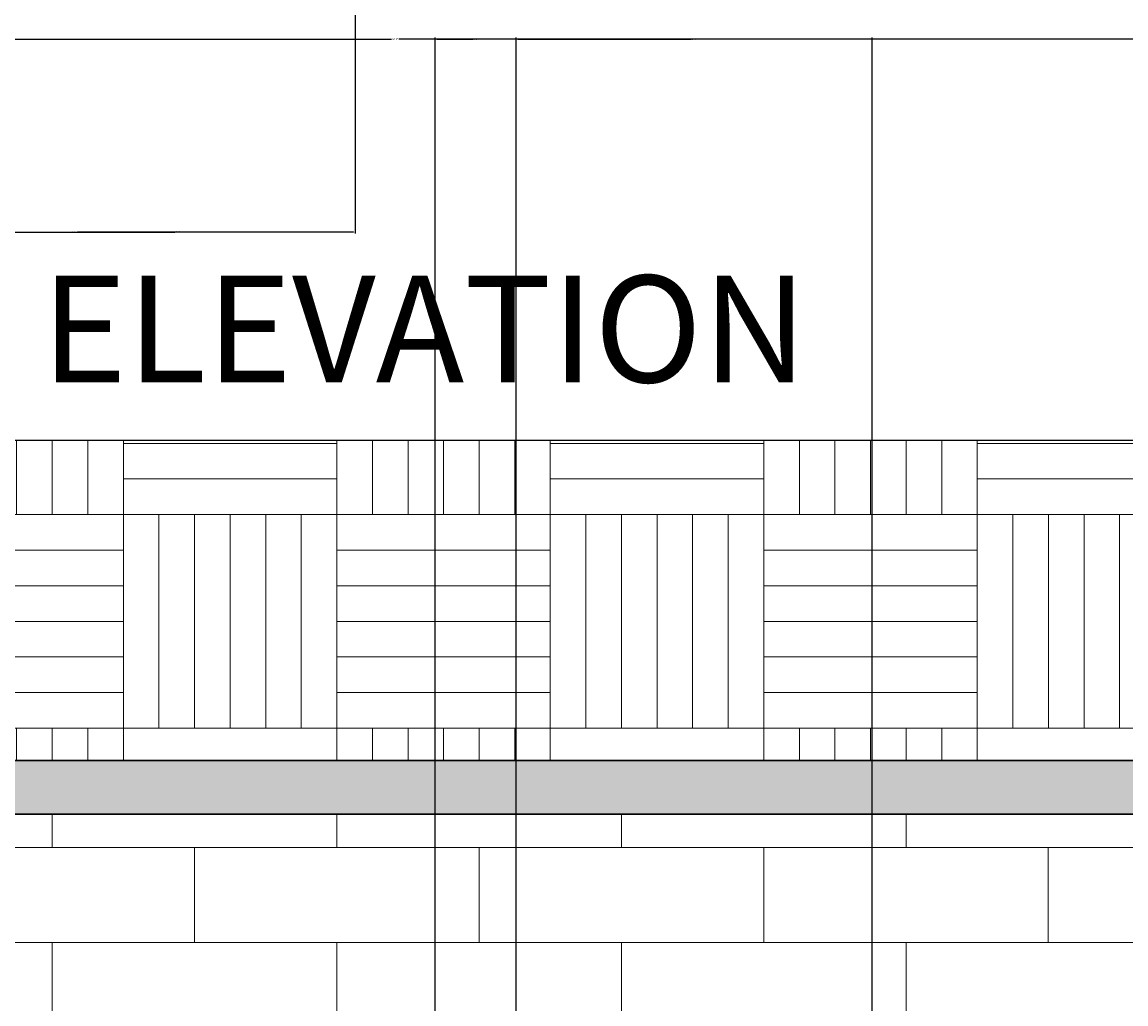
# Model space of a CAD drawing. Units: inches. Extents: x 37 to 824, y -700 to 234.
# Tile 20 of 77: x 253 to 377, y -487 to -377. Entities that reach past the tile are written whole.
import ezdxf

# ---------------------------------------------------------------- set-up
doc = ezdxf.new("R2010")
doc.units = ezdxf.units.IN
doc.header["$MEASUREMENT"] = 0
for name, color, linetype, lineweight in [('A-ANNO-DIMS', 2, 'Continuous', 18), ('A-ANNO-TEXT', 7, 'Continuous', 18), ('A-ELEV', 3, 'Continuous', 25), ('A-ELEV-PATT', 8, 'Continuous', 13)]:
    doc.layers.add(name, color=color, linetype=linetype, lineweight=lineweight)
doc.styles.get("Standard").update_dxf_attribs({"font": 'arial.ttf'})
doc.dimstyles.get("Standard").update_dxf_attribs({"dimtxt": 0.18, "dimasz": 0.18, "dimexe": 0.18, "dimexo": 0.0625, "dimgap": 0.09, "dimtad": 0, "dimtih": 1, "dimtoh": 1, "dimdec": 1, "dimzin": 0, "dimdsep": 46, "dimlunit": 4, "dimtxsty": 'Standard', "dimcen": 0.09, "dimadec": 0, "dimazin": 0, "dimtfac": 1, "dimtdec": 1, "dimtofl": 0, "dimtmove": 0, "dimatfit": 3, "dimfxl": 1, "dimtolj": 1, "dimtzin": 0, "dimarcsym": 0})

# ---------------------------------------------------------------- blocks, each defined once
blk = doc.blocks.new('*D66')
at = {"layer": 'A-ANNO-DIMS', "color": 0, "lineweight": -2, "ltscale": 0.5, "transparency": 16777216}
for p, q in [((161.08, -423.56), (161.08, -378.38)), ((428.08, -423.56), (428.08, -378.38)), ((161.26, -378.56), (294.18, -378.56)), ((427.9, -378.56), (294.98, -378.56))]:
    blk.add_line(p, q, dxfattribs=at)
at = {"layer": 'A-ANNO-DIMS', "color": 0, "ltscale": 0.5, "transparency": 16777216}
for points in [[(161.26, -378.53), (161.26, -378.59), (161.08, -378.56)], [(427.9, -378.53), (427.9, -378.59), (428.08, -378.56)]]:
    blk.add_solid(points, dxfattribs=at)
at = {"layer": 'Defpoints', "color": 0, "ltscale": 0.5, "transparency": 16777216}
for p in [(428.08, -378.56), (161.08, -423.63), (428.08, -423.63)]:
    blk.add_point(p, dxfattribs=at)
at = {"layer": 'A-ANNO-DIMS', "color": 0, "ltscale": 0.5, "transparency": 16777216, "insert": (294.58, -378.56), "char_height": 0.18, "attachment_point": 5}
blk.add_mtext('\\A1;22\'-3"', dxfattribs=at)
blk = doc.blocks.new('*D77')
at = {"layer": 'A-ANNO-DIMS', "color": 0, "lineweight": -2, "ltscale": 0.5, "transparency": 16777216}
for p, q in [((227.08, 45.5), (227.08, -400.41)), ((290.08, 15.03), (290.08, -400.41)), ((227.26, -400.23), (258.25, -400.23)), ((289.9, -400.23), (258.91, -400.23))]:
    blk.add_line(p, q, dxfattribs=at)
at = {"layer": 'A-ANNO-DIMS', "color": 0, "ltscale": 0.5, "transparency": 16777216}
for points in [[(227.26, -400.2), (227.26, -400.26), (227.08, -400.23)], [(289.9, -400.2), (289.9, -400.26), (290.08, -400.23)]]:
    blk.add_solid(points, dxfattribs=at)
at = {"layer": 'Defpoints', "color": 0, "ltscale": 0.5, "transparency": 16777216}
for p in [(227.08, 45.56), (290.08, 15.09), (290.08, -400.23)]:
    blk.add_point(p, dxfattribs=at)
at = {"layer": 'A-ANNO-DIMS', "color": 0, "ltscale": 0.5, "transparency": 16777216, "insert": (258.58, -400.23), "char_height": 0.18, "attachment_point": 5}
blk.add_mtext('\\A1;5\'-3"', dxfattribs=at)
blk = doc.blocks.new('*D81')
at = {"layer": 'A-ANNO-DIMS', "color": 0, "lineweight": -2, "ltscale": 0.5, "transparency": 16777216}
for p, q in [((290.08, -164.97), (290.08, -400.41)), ((250.19, -167.97), (250.19, -400.41)), ((250.37, -400.23), (269.8, -400.23)), ((289.9, -400.23), (270.46, -400.23))]:
    blk.add_line(p, q, dxfattribs=at)
at = {"layer": 'A-ANNO-DIMS', "color": 0, "ltscale": 0.5, "transparency": 16777216}
for points in [[(250.37, -400.2), (250.37, -400.26), (250.19, -400.23)], [(289.9, -400.2), (289.9, -400.26), (290.08, -400.23)]]:
    blk.add_solid(points, dxfattribs=at)
at = {"layer": 'Defpoints', "color": 0, "ltscale": 0.5, "transparency": 16777216}
for p in [(290.08, -164.91), (250.19, -167.91), (290.08, -400.23)]:
    blk.add_point(p, dxfattribs=at)
at = {"layer": 'A-ANNO-DIMS', "color": 0, "ltscale": 0.5, "transparency": 16777216, "insert": (270.13, -400.23), "char_height": 0.18, "attachment_point": 5}
blk.add_mtext('\\A1;3\'-4"', dxfattribs=at)
blk = doc.blocks.new('*D98')
at = {"layer": 'A-ANNO-DIMS', "color": 0, "lineweight": -2, "ltscale": 0.5, "transparency": 16777216}
for p, q in [((299.08, -489.56), (299.08, -378.38)), ((308.2, -495.94), (308.2, -378.38)), ((299.26, -378.56), (303.31, -378.56)), ((308.02, -378.56), (303.97, -378.56))]:
    blk.add_line(p, q, dxfattribs=at)
at = {"layer": 'A-ANNO-DIMS', "color": 0, "ltscale": 0.5, "transparency": 16777216}
for points in [[(299.26, -378.53), (299.26, -378.59), (299.08, -378.56)], [(308.02, -378.53), (308.02, -378.59), (308.2, -378.56)]]:
    blk.add_solid(points, dxfattribs=at)
at = {"layer": 'Defpoints', "color": 0, "ltscale": 0.5, "transparency": 16777216}
for p in [(308.2, -378.56), (299.08, -489.63), (308.2, -496.01)]:
    blk.add_point(p, dxfattribs=at)
at = {"layer": 'A-ANNO-DIMS', "color": 0, "ltscale": 0.5, "transparency": 16777216, "insert": (303.64, -378.56), "char_height": 0.18, "attachment_point": 5}
blk.add_mtext('\\A1;0\'-9"', dxfattribs=at)
blk = doc.blocks.new('*D99')
at = {"layer": 'A-ANNO-DIMS', "color": 0, "lineweight": -2, "ltscale": 0.5, "transparency": 16777216}
for p, q in [((308.2, -495.94), (308.2, -378.38)), ((348.2, -495.94), (348.2, -378.38)), ((308.38, -378.56), (327.87, -378.56)), ((348.02, -378.56), (328.52, -378.56))]:
    blk.add_line(p, q, dxfattribs=at)
at = {"layer": 'A-ANNO-DIMS', "color": 0, "ltscale": 0.5, "transparency": 16777216}
for points in [[(308.38, -378.53), (308.38, -378.59), (308.2, -378.56)], [(348.02, -378.53), (348.02, -378.59), (348.2, -378.56)]]:
    blk.add_solid(points, dxfattribs=at)
at = {"layer": 'Defpoints', "color": 0, "ltscale": 0.5, "transparency": 16777216}
for p in [(348.2, -378.56), (308.2, -496.01), (348.2, -496.01)]:
    blk.add_point(p, dxfattribs=at)
at = {"layer": 'A-ANNO-DIMS', "color": 0, "ltscale": 0.5, "transparency": 16777216, "insert": (328.2, -378.56), "char_height": 0.18, "attachment_point": 5}
blk.add_mtext('\\A1;3\'-4"', dxfattribs=at)

msp = doc.modelspace()

# ---------------------------------------------------------------- hatches: boundary and pattern name
at = {"layer": 'A-ELEV-PATT', "ltscale": 0.5}
h = msp.add_hatch(dxfattribs=at)
h.set_pattern_fill('AR-PARQ1', color=256, scale=2)
h.paths.add_polyline_path([(428.08, -423.63), (161.08, -423.63), (161.08, -459.63), (428.08, -459.63)])
h = msp.add_hatch(color=256, dxfattribs=at)
h.dxf.hatch_style = 1
h.paths.add_polyline_path([(161.08, -459.63), (161.08, -465.63), (428.08, -465.63), (428.08, -459.63)])
h.paths.add_polyline_path([(229.03, -498.21), (214.53, -498.21), (214.53, -529.21), (229.03, -529.21)])
h.paths.add_polyline_path([(245.53, -498.21), (230.03, -498.21), (230.03, -529.21), (245.53, -529.21)])
h.paths.add_polyline_path([(315.2, -574.01), (341.2, -574.01), (341.2, -505.03), (315.2, -505.03)])
h = msp.add_hatch(dxfattribs=at)
h.set_pattern_fill('AR-BRSTD', color=256, scale=4)
h.paths.add_polyline_path([(299.08, -489.63), (358.13, -489.63), (358.13, -585.63), (428.08, -585.63), (428.08, -465.63), (161.08, -465.63), (161.08, -585.63), (299.08, -585.63)])
h.paths.add_polyline_path([(205.08, -537.63), (205.08, -489.63), (255.08, -489.63), (255.08, -537.63)], flags=16)

# ---------------------------------------------------------------- linework, layer by layer
at = {"layer": 'A-ELEV', "ltscale": 0.5}
for points in [[(161.08, -423.63), (428.08, -423.63), (428.08, -459.63), (161.08, -459.63)], [(161.08, -459.63), (428.08, -459.63), (428.08, -465.63), (161.08, -465.63)], [(161.08, -465.63), (428.08, -465.63), (428.08, -585.63), (161.08, -585.63)]]:
    msp.add_lwpolyline(points, close=True, dxfattribs=at)

# ---------------------------------------------------------------- texts
at = {"layer": 'A-ANNO-TEXT'}
msp.add_text('ELEVATION', height=12, dxfattribs=at).set_placement((254.8, -417.12))

# ---------------------------------------------------------------- dimensions: what is measured, and where the dimension line sits
at = {"layer": 'A-ANNO-DIMS', "ltscale": 0.5}
for base, p1, p2, picture, middle in [((290.08, -400.23), (227.08, 45.56), (290.08, 15.09), '*D77', (258.58, -400.23)), ((290.08, -400.23), (250.19, -167.91), (290.08, -164.91), '*D81', (270.13, -400.23)), ((428.08, -378.56), (161.08, -423.63), (428.08, -423.63), '*D66', (294.58, -378.56)), ((308.2, -378.56), (299.08, -489.63), (308.2, -496.01), '*D98', (303.64, -378.56)), ((348.2, -378.56), (308.2, -496.01), (348.2, -496.01), '*D99', (328.2, -378.56))]:
    dim = msp.add_linear_dim(base=base, p1=p1, p2=p2, dimstyle='Standard', override={"dimdec": 1, "dimlfac": 1, "dimrnd": 0, "dimzin": 1, "dimdsep": 46, "dimlunit": 4, "dimfrac": 2}, dxfattribs=at)
    dim.commit()
    dim.dimension.update_dxf_attribs({"geometry": picture, "text_midpoint": middle})

doc.saveas('drawing.dxf')
